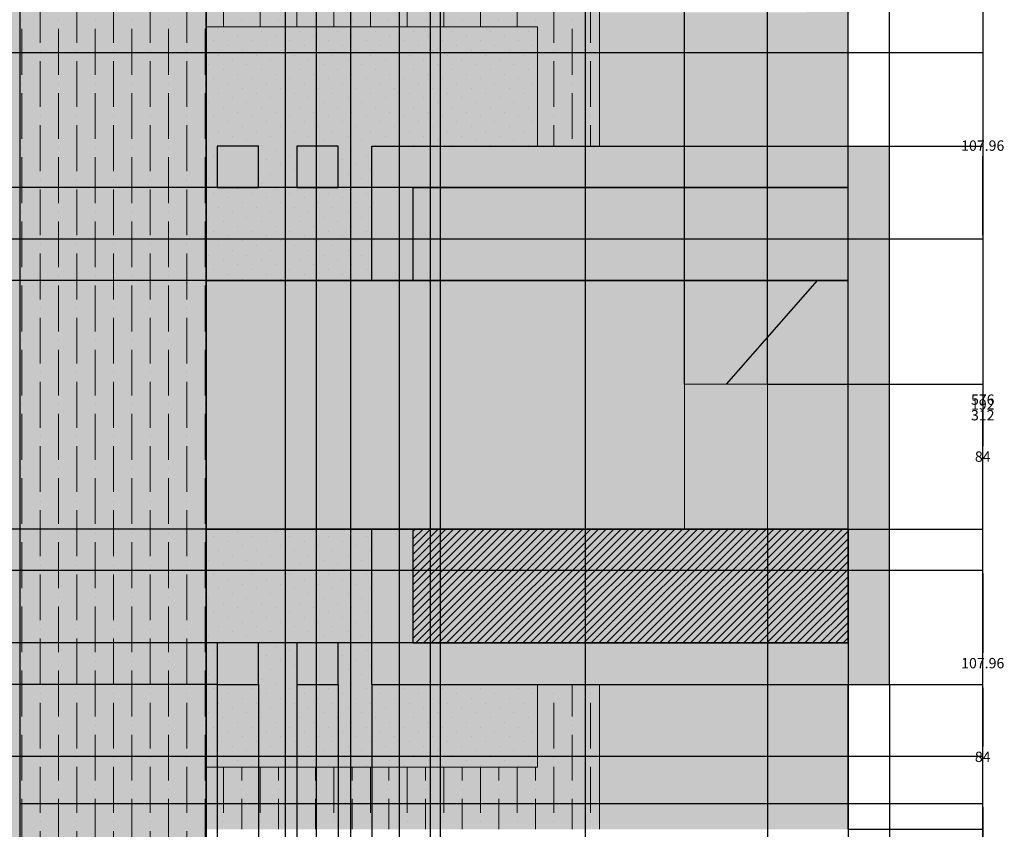
# Model space of a CAD drawing. Units: inches. Extents: x 180 to 1069, y 71 to 1267.
# Tile 7 of 8: x 498 to 1069, y 474 to 943. Entities that reach past the tile are written whole.
import ezdxf

# ---------------------------------------------------------------- set-up
doc = ezdxf.new("R2010")
doc.units = ezdxf.units.IN
doc.header["$MEASUREMENT"] = 0
for name, color, linetype, lineweight in [('A-ANNO-DIMS', 2, 'Continuous', 18), ('A-DOOR', 7, 'Continuous', 20), ('A-DOOR-PANL-PATT', 25, 'Continuous', 13), ('A-ELEV-FRAM', 7, 'Continuous', 25), ('A-RAIL-GLAS-DIAG-PATT', 140, 'Continuous', 13), ('A-WALL', 7, 'Continuous', 30), ('A-WALL-CLAD', 7, 'Continuous', 18), ('A-WALL-SCRN-JNTS-PATT', 8, 'Continuous', 13)]:
    doc.layers.add(name, color=color, linetype=linetype, lineweight=lineweight)
for name, color, linetype, lineweight, true_color in [('A-ELEV-BAND-PATT', 30, 'Continuous', 13, 0xf26722), ('A-ELEV-FRAM-PATT', 53, 'Continuous', 13, 0xefd648), ('A-ELEV-REVL-PATT', 9, 'Continuous', 13, 0xc7c8ca), ('A-RAIL-GLAS-PATT', 253, 'Continuous', 13, 0x9f9f8e), ('A-WALL-PANL-PATT', 252, 'Continuous', 13, 0x939598), ('A-WALL-PATT', 253, 'Continuous', 13, 0x9f9f8e), ('A-WALL-SCRN-PATT', 251, 'Continuous', 13, 0x636466), ('A-WALL-STUC-PATT', 9, 'Continuous', 13, 0xc7c8ca)]:
    doc.layers.add(name, color=color, linetype=linetype, lineweight=lineweight, true_color=true_color)
doc.styles.get("Standard").update_dxf_attribs({"font": 'arial.ttf'})
doc.dimstyles.get("Standard").update_dxf_attribs({"dimtxt": 6, "dimasz": 2, "dimexe": 0.18, "dimexo": 0.0625, "dimgap": 3, "dimtad": 0, "dimtih": 1, "dimtoh": 1, "dimdec": 0, "dimzin": 0, "dimdsep": 46, "dimlunit": 3, "dimtxsty": 'Standard', "dimcen": 0.09, "dimadec": 0, "dimazin": 0, "dimtfac": 1, "dimtdec": 0, "dimtofl": 0, "dimtmove": 0, "dimatfit": 3, "dimfxl": 1, "dimtolj": 1, "dimtzin": 0, "dimarcsym": 0})

# ---------------------------------------------------------------- blocks, each defined once
blk = doc.blocks.new('FACADE-SQUARE-INSET')
blk.add_lwpolyline([(24, 24), (0, 24), (0, 0), (24, 0)], close=True)
blk = doc.blocks.new('*D38')
at = {"layer": 'A-ANNO-DIMS', "color": 0, "lineweight": -2, "transparency": 16777216}
for p, q in [((978.15, 473.82), (1056.28, 473.82)), ((1056.1, 471.82), (1056.1, 415.94)), ((1056.1, 348.05), (1056.1, 403.92)), ((978.15, 346.05), (1056.28, 346.05))]:
    blk.add_line(p, q, dxfattribs=at)
at = {"layer": 'A-ANNO-DIMS', "color": 0, "transparency": 16777216}
for points in [[(1055.77, 471.82), (1056.43, 471.82), (1056.1, 473.82)], [(1055.77, 348.05), (1056.43, 348.05), (1056.1, 346.05)]]:
    blk.add_solid(points, dxfattribs=at)
at = {"layer": 'Defpoints', "color": 0, "transparency": 16777216}
for p in [(978.09, 473.82), (1056.1, 473.82), (978.09, 346.05)]:
    blk.add_point(p, dxfattribs=at)
at = {"layer": 'A-ANNO-DIMS', "color": 0, "transparency": 16777216, "insert": (1056.1, 409.93), "char_height": 6, "attachment_point": 5}
blk.add_mtext('\\A1;127.77', dxfattribs=at)
blk = doc.blocks.new('*D40')
at = {"layer": 'A-ANNO-DIMS', "color": 0, "lineweight": -2, "transparency": 16777216}
for p, q in [((652.09, 338.11), (652.09, 1263.01)), ((654.09, 1262.83), (686.8, 1262.83)), ((734.09, 1262.83), (701.38, 1262.83)), ((736.09, 338.11), (736.09, 1263.01))]:
    blk.add_line(p, q, dxfattribs=at)
at = {"layer": 'A-ANNO-DIMS', "color": 0, "transparency": 16777216}
for points in [[(654.09, 1263.16), (654.09, 1262.5), (652.09, 1262.83)], [(734.09, 1263.16), (734.09, 1262.5), (736.09, 1262.83)]]:
    blk.add_solid(points, dxfattribs=at)
at = {"layer": 'Defpoints', "color": 0, "transparency": 16777216}
for p in [(736.09, 1262.83), (652.09, 338.05), (736.09, 338.05)]:
    blk.add_point(p, dxfattribs=at)
at = {"layer": 'A-ANNO-DIMS', "color": 0, "transparency": 16777216, "insert": (694.09, 1262.83), "char_height": 6, "attachment_point": 5}
blk.add_mtext('\\A1;84', dxfattribs=at)
blk = doc.blocks.new('*D42')
at = {"layer": 'A-ANNO-DIMS', "color": 0, "lineweight": -2, "transparency": 16777216}
for p, q in [((670.09, 301.11), (670.09, 1263.01)), ((672.09, 1262.83), (686.66, 1262.83)), ((716.09, 1262.83), (701.51, 1262.83)), ((718.09, 301.11), (718.09, 1263.01))]:
    blk.add_line(p, q, dxfattribs=at)
at = {"layer": 'A-ANNO-DIMS', "color": 0, "transparency": 16777216}
for points in [[(672.09, 1263.16), (672.09, 1262.5), (670.09, 1262.83)], [(716.09, 1263.16), (716.09, 1262.5), (718.09, 1262.83)]]:
    blk.add_solid(points, dxfattribs=at)
at = {"layer": 'Defpoints', "color": 0, "transparency": 16777216}
for p in [(718.09, 1262.83), (670.09, 301.05), (718.09, 301.05)]:
    blk.add_point(p, dxfattribs=at)
at = {"layer": 'A-ANNO-DIMS', "color": 0, "transparency": 16777216, "insert": (694.09, 1262.83), "char_height": 6, "attachment_point": 5}
blk.add_mtext('\\A1;48', dxfattribs=at)
blk = doc.blocks.new('*D44')
at = {"layer": 'A-ANNO-DIMS', "color": 0, "lineweight": -2, "transparency": 16777216}
for p, q in [((606.09, 442.3), (606.09, 1263.01)), ((608.09, 1262.83), (635.5, 1262.83)), ((688, 1262.83), (660.59, 1262.83)), ((690, 442.3), (690, 1263.01))]:
    blk.add_line(p, q, dxfattribs=at)
at = {"layer": 'A-ANNO-DIMS', "color": 0, "transparency": 16777216}
for points in [[(608.09, 1263.16), (608.09, 1262.5), (606.09, 1262.83)], [(688, 1263.16), (688, 1262.5), (690, 1262.83)]]:
    blk.add_solid(points, dxfattribs=at)
at = {"layer": 'Defpoints', "color": 0, "transparency": 16777216}
for p in [(690, 1262.83), (606.09, 442.24), (690, 442.24)]:
    blk.add_point(p, dxfattribs=at)
at = {"layer": 'A-ANNO-DIMS', "color": 0, "transparency": 16777216, "insert": (648.04, 1262.83), "char_height": 6, "attachment_point": 5}
blk.add_mtext('\\A1;83.91', dxfattribs=at)
blk = doc.blocks.new('*D45')
at = {"layer": 'A-ANNO-DIMS', "color": 0, "lineweight": -2, "transparency": 16777216}
for p, q in [((690, 442.3), (690, 1263.01)), ((692, 1262.83), (702.82, 1262.83)), ((739.89, 1262.83), (729.08, 1262.83)), ((741.89, 442.3), (741.89, 1263.01))]:
    blk.add_line(p, q, dxfattribs=at)
at = {"layer": 'A-ANNO-DIMS', "color": 0, "transparency": 16777216}
for points in [[(692, 1263.16), (692, 1262.5), (690, 1262.83)], [(739.89, 1263.16), (739.89, 1262.5), (741.89, 1262.83)]]:
    blk.add_solid(points, dxfattribs=at)
at = {"layer": 'Defpoints', "color": 0, "transparency": 16777216}
for p in [(741.89, 1262.83), (690, 442.24), (741.89, 442.24)]:
    blk.add_point(p, dxfattribs=at)
at = {"layer": 'A-ANNO-DIMS', "color": 0, "transparency": 16777216, "insert": (715.95, 1262.83), "char_height": 6, "attachment_point": 5}
blk.add_mtext('\\A1;51.89', dxfattribs=at)
blk = doc.blocks.new('*D46')
at = {"layer": 'A-ANNO-DIMS', "color": 0, "lineweight": -2, "transparency": 16777216}
for p, q in [((741.89, 442.3), (741.89, 1263.01)), ((743.89, 1262.83), (776.6, 1262.83)), ((823.89, 1262.83), (791.18, 1262.83)), ((825.89, 442.3), (825.89, 1263.01))]:
    blk.add_line(p, q, dxfattribs=at)
at = {"layer": 'A-ANNO-DIMS', "color": 0, "transparency": 16777216}
for points in [[(743.89, 1263.16), (743.89, 1262.5), (741.89, 1262.83)], [(823.89, 1263.16), (823.89, 1262.5), (825.89, 1262.83)]]:
    blk.add_solid(points, dxfattribs=at)
at = {"layer": 'Defpoints', "color": 0, "transparency": 16777216}
for p in [(825.89, 1262.83), (741.89, 442.24), (825.89, 442.24)]:
    blk.add_point(p, dxfattribs=at)
at = {"layer": 'A-ANNO-DIMS', "color": 0, "transparency": 16777216, "insert": (783.89, 1262.83), "char_height": 6, "attachment_point": 5}
blk.add_mtext('\\A1;84', dxfattribs=at)
blk = doc.blocks.new('*D53')
at = {"layer": 'A-ANNO-DIMS', "color": 0, "lineweight": -2, "transparency": 16777216}
for p, q in [((438.15, 624.07), (1056.28, 624.07)), ((1056.1, 622.07), (1056.1, 576.16)), ((1056.1, 518.12), (1056.1, 564.03)), ((467.25, 516.12), (1056.28, 516.12))]:
    blk.add_line(p, q, dxfattribs=at)
at = {"layer": 'A-ANNO-DIMS', "color": 0, "transparency": 16777216}
for points in [[(1055.77, 622.07), (1056.43, 622.07), (1056.1, 624.07)], [(1055.77, 518.12), (1056.43, 518.12), (1056.1, 516.12)]]:
    blk.add_solid(points, dxfattribs=at)
at = {"layer": 'Defpoints', "color": 0, "transparency": 16777216}
for p in [(438.09, 624.07), (1056.1, 624.07), (467.19, 516.12)]:
    blk.add_point(p, dxfattribs=at)
at = {"layer": 'A-ANNO-DIMS', "color": 0, "transparency": 16777216, "insert": (1056.1, 570.1), "char_height": 6, "attachment_point": 5}
blk.add_mtext('\\A1;107.96', dxfattribs=at)
blk = doc.blocks.new('*D54')
at = {"layer": 'A-ANNO-DIMS', "color": 0, "lineweight": -2, "transparency": 16777216}
for p, q in [((438.15, 816.07), (1056.28, 816.07)), ((1056.1, 814.07), (1056.1, 726.14)), ((1056.1, 626.07), (1056.1, 714.01)), ((438.15, 624.07), (1056.28, 624.07))]:
    blk.add_line(p, q, dxfattribs=at)
at = {"layer": 'A-ANNO-DIMS', "color": 0, "transparency": 16777216}
for points in [[(1055.77, 814.07), (1056.43, 814.07), (1056.1, 816.07)], [(1055.77, 626.07), (1056.43, 626.07), (1056.1, 624.07)]]:
    blk.add_solid(points, dxfattribs=at)
at = {"layer": 'Defpoints', "color": 0, "transparency": 16777216}
for p in [(438.09, 816.07), (1056.1, 816.07), (438.09, 624.07)]:
    blk.add_point(p, dxfattribs=at)
at = {"layer": 'A-ANNO-DIMS', "color": 0, "transparency": 16777216, "insert": (1056.1, 720.07), "char_height": 6, "attachment_point": 5}
blk.add_mtext('\\A1;192', dxfattribs=at)
blk = doc.blocks.new('*D55')
at = {"layer": 'A-ANNO-DIMS', "color": 0, "lineweight": -2, "transparency": 16777216}
for p, q in [((467.25, 924.03), (1056.28, 924.03)), ((1056.1, 922.03), (1056.1, 876.12)), ((1056.1, 818.07), (1056.1, 863.99)), ((438.15, 816.07), (1056.28, 816.07))]:
    blk.add_line(p, q, dxfattribs=at)
at = {"layer": 'A-ANNO-DIMS', "color": 0, "transparency": 16777216}
for points in [[(1055.77, 922.03), (1056.43, 922.03), (1056.1, 924.03)], [(1055.77, 818.07), (1056.43, 818.07), (1056.1, 816.07)]]:
    blk.add_solid(points, dxfattribs=at)
at = {"layer": 'Defpoints', "color": 0, "transparency": 16777216}
for p in [(467.19, 924.03), (1056.1, 924.03), (438.09, 816.07)]:
    blk.add_point(p, dxfattribs=at)
at = {"layer": 'A-ANNO-DIMS', "color": 0, "transparency": 16777216, "insert": (1056.1, 870.05), "char_height": 6, "attachment_point": 5}
blk.add_mtext('\\A1;107.96', dxfattribs=at)
blk = doc.blocks.new('*D58')
at = {"layer": 'A-ANNO-DIMS', "color": 0, "lineweight": -2, "transparency": 16777216}
for p, q in [((606.09, 1010.75), (606.09, 74.62)), ((498.09, 956.75), (498.09, 74.62)), ((500.09, 74.8), (542.74, 74.8)), ((604.09, 74.8), (561.44, 74.8))]:
    blk.add_line(p, q, dxfattribs=at)
at = {"layer": 'A-ANNO-DIMS', "color": 0, "transparency": 16777216}
for points in [[(500.09, 75.14), (500.09, 74.47), (498.09, 74.8)], [(604.09, 75.14), (604.09, 74.47), (606.09, 74.8)]]:
    blk.add_solid(points, dxfattribs=at)
at = {"layer": 'Defpoints', "color": 0, "transparency": 16777216}
for p in [(606.09, 1010.82), (498.09, 956.82), (606.09, 74.8)]:
    blk.add_point(p, dxfattribs=at)
at = {"layer": 'A-ANNO-DIMS', "color": 0, "transparency": 16777216, "insert": (552.09, 74.8), "char_height": 6, "attachment_point": 5}
blk.add_mtext('\\A1;108', dxfattribs=at)
blk = doc.blocks.new('*D59')
at = {"layer": 'A-ANNO-DIMS', "color": 0, "lineweight": -2, "transparency": 16777216}
for p, q in [((606.15, 1010.82), (1056.28, 1010.82)), ((1056.1, 1008.82), (1056.1, 728.88)), ((1056.1, 436.82), (1056.1, 716.75)), ((606.15, 434.82), (1056.28, 434.82))]:
    blk.add_line(p, q, dxfattribs=at)
at = {"layer": 'A-ANNO-DIMS', "color": 0, "transparency": 16777216}
for points in [[(1055.77, 1008.82), (1056.43, 1008.82), (1056.1, 1010.82)], [(1055.77, 436.82), (1056.43, 436.82), (1056.1, 434.82)]]:
    blk.add_solid(points, dxfattribs=at)
at = {"layer": 'Defpoints', "color": 0, "transparency": 16777216}
for p in [(606.09, 1010.82), (1056.1, 1010.82), (606.09, 434.82)]:
    blk.add_point(p, dxfattribs=at)
at = {"layer": 'A-ANNO-DIMS', "color": 0, "transparency": 16777216, "insert": (1056.1, 722.82), "char_height": 6, "attachment_point": 5}
blk.add_mtext('\\A1;576', dxfattribs=at)
blk = doc.blocks.new('*D60')
at = {"layer": 'A-ANNO-DIMS', "color": 0, "lineweight": -2, "transparency": 16777216}
for p, q in [((498.15, 488.82), (1056.28, 488.82)), ((1056.1, 486.82), (1056.1, 467.87)), ((1056.1, 436.82), (1056.1, 455.76)), ((606.15, 434.82), (1056.28, 434.82))]:
    blk.add_line(p, q, dxfattribs=at)
at = {"layer": 'A-ANNO-DIMS', "color": 0, "transparency": 16777216}
for points in [[(1055.77, 486.82), (1056.43, 486.82), (1056.1, 488.82)], [(1055.77, 436.82), (1056.43, 436.82), (1056.1, 434.82)]]:
    blk.add_solid(points, dxfattribs=at)
at = {"layer": 'Defpoints', "color": 0, "transparency": 16777216}
for p in [(498.09, 488.82), (606.09, 434.82), (1056.1, 434.82)]:
    blk.add_point(p, dxfattribs=at)
at = {"layer": 'A-ANNO-DIMS', "color": 0, "transparency": 16777216, "insert": (1056.1, 461.82), "char_height": 6, "attachment_point": 5}
blk.add_mtext('\\A1;54', dxfattribs=at)
blk = doc.blocks.new('*D64')
at = {"layer": 'A-ANNO-DIMS', "color": 0, "lineweight": -2, "transparency": 16777216}
for p, q in [((612.46, 845.82), (191.89, 845.82)), ((192.07, 843.82), (192.07, 707.88)), ((192.07, 559.82), (192.07, 695.75)), ((612.46, 557.82), (191.89, 557.82))]:
    blk.add_line(p, q, dxfattribs=at)
at = {"layer": 'A-ANNO-DIMS', "color": 0, "transparency": 16777216}
for points in [[(191.74, 843.82), (192.41, 843.82), (192.07, 845.82)], [(191.74, 559.82), (192.41, 559.82), (192.07, 557.82)]]:
    blk.add_solid(points, dxfattribs=at)
at = {"layer": 'Defpoints', "color": 0, "transparency": 16777216}
for p in [(192.07, 845.82), (612.53, 845.82), (612.53, 557.82)]:
    blk.add_point(p, dxfattribs=at)
at = {"layer": 'A-ANNO-DIMS', "color": 0, "transparency": 16777216, "insert": (192.07, 701.82), "char_height": 6, "attachment_point": 5}
blk.add_mtext('\\A1;288', dxfattribs=at)
blk = doc.blocks.new('*D65')
at = {"layer": 'A-ANNO-DIMS', "color": 0, "lineweight": -2, "transparency": 16777216}
for p, q in [((636.53, 557.75), (636.53, 74.62)), ((658.66, 557.75), (658.66, 74.62)), ((638.53, 74.8), (656.66, 74.8)), ((658.66, 74.8), (660.66, 74.8))]:
    blk.add_line(p, q, dxfattribs=at)
at = {"layer": 'A-ANNO-DIMS', "color": 0, "transparency": 16777216}
for points in [[(638.53, 75.14), (638.53, 74.47), (636.53, 74.8)], [(656.66, 75.14), (656.66, 74.47), (658.66, 74.8)]]:
    blk.add_solid(points, dxfattribs=at)
at = {"layer": 'Defpoints', "color": 0, "transparency": 16777216}
for p in [(636.53, 557.82), (658.66, 557.82), (658.66, 74.8)]:
    blk.add_point(p, dxfattribs=at)
at = {"layer": 'A-ANNO-DIMS', "color": 0, "transparency": 16777216, "insert": (676.17, 74.8), "char_height": 6, "attachment_point": 5}
blk.add_mtext('\\A1;22.133', dxfattribs=at)
blk = doc.blocks.new('*D66')
at = {"layer": 'A-ANNO-DIMS', "color": 0, "lineweight": -2, "transparency": 16777216}
for p, q in [((606.09, 647.75), (606.09, 74.62)), ((612.53, 557.75), (612.53, 74.62)), ((604.09, 74.8), (602.09, 74.8)), ((614.53, 74.8), (616.53, 74.8))]:
    blk.add_line(p, q, dxfattribs=at)
at = {"layer": 'A-ANNO-DIMS', "color": 0, "transparency": 16777216}
for points in [[(604.09, 75.14), (604.09, 74.47), (606.09, 74.8)], [(614.53, 75.14), (614.53, 74.47), (612.53, 74.8)]]:
    blk.add_solid(points, dxfattribs=at)
at = {"layer": 'Defpoints', "color": 0, "transparency": 16777216}
for p in [(606.09, 647.82), (612.53, 557.82), (612.53, 74.8)]:
    blk.add_point(p, dxfattribs=at)
at = {"layer": 'A-ANNO-DIMS', "color": 0, "transparency": 16777216, "insert": (627.32, 74.8), "char_height": 6, "attachment_point": 5}
blk.add_mtext('\\A1;6.44', dxfattribs=at)
blk = doc.blocks.new('*D67')
at = {"layer": 'A-ANNO-DIMS', "color": 0, "lineweight": -2, "transparency": 16777216}
for p, q in [((682.66, 557.75), (682.66, 74.62)), ((702.09, 557.75), (702.09, 74.62)), ((684.66, 74.8), (700.09, 74.8)), ((702.09, 74.8), (704.09, 74.8))]:
    blk.add_line(p, q, dxfattribs=at)
at = {"layer": 'A-ANNO-DIMS', "color": 0, "transparency": 16777216}
for points in [[(684.66, 75.14), (684.66, 74.47), (682.66, 74.8)], [(700.09, 75.14), (700.09, 74.47), (702.09, 74.8)]]:
    blk.add_solid(points, dxfattribs=at)
at = {"layer": 'Defpoints', "color": 0, "transparency": 16777216}
for p in [(682.66, 557.82), (702.09, 557.82), (702.09, 74.8)]:
    blk.add_point(p, dxfattribs=at)
at = {"layer": 'A-ANNO-DIMS', "color": 0, "transparency": 16777216, "insert": (719.26, 74.8), "char_height": 6, "attachment_point": 5}
blk.add_mtext('\\A1;19.427', dxfattribs=at)
blk = doc.blocks.new('*D68')
at = {"layer": 'A-ANNO-DIMS', "color": 0, "lineweight": -2, "transparency": 16777216}
for p, q in [((702.09, 557.75), (702.09, 74.62)), ((1002.09, 557.75), (1002.09, 74.62)), ((704.09, 74.8), (842.47, 74.8)), ((1000.09, 74.8), (861.7, 74.8))]:
    blk.add_line(p, q, dxfattribs=at)
at = {"layer": 'A-ANNO-DIMS', "color": 0, "transparency": 16777216}
for points in [[(704.09, 75.14), (704.09, 74.47), (702.09, 74.8)], [(1000.09, 75.14), (1000.09, 74.47), (1002.09, 74.8)]]:
    blk.add_solid(points, dxfattribs=at)
at = {"layer": 'Defpoints', "color": 0, "transparency": 16777216}
for p in [(702.09, 557.82), (1002.09, 557.82), (1002.09, 74.8)]:
    blk.add_point(p, dxfattribs=at)
at = {"layer": 'A-ANNO-DIMS', "color": 0, "transparency": 16777216, "insert": (852.09, 74.8), "char_height": 6, "attachment_point": 5}
blk.add_mtext('\\A1;300', dxfattribs=at)
blk = doc.blocks.new('*D69')
at = {"layer": 'A-ANNO-DIMS', "color": 0, "lineweight": -2, "transparency": 16777216}
for p, q in [((1002.15, 557.82), (1056.28, 557.82)), ((1056.1, 555.82), (1056.1, 521.88)), ((1056.1, 475.82), (1056.1, 509.75)), ((978.15, 473.82), (1056.28, 473.82))]:
    blk.add_line(p, q, dxfattribs=at)
at = {"layer": 'A-ANNO-DIMS', "color": 0, "transparency": 16777216}
for points in [[(1055.77, 555.82), (1056.43, 555.82), (1056.1, 557.82)], [(1055.77, 475.82), (1056.43, 475.82), (1056.1, 473.82)]]:
    blk.add_solid(points, dxfattribs=at)
at = {"layer": 'Defpoints', "color": 0, "transparency": 16777216}
for p in [(1002.09, 557.82), (1056.1, 557.82), (978.09, 473.82)]:
    blk.add_point(p, dxfattribs=at)
at = {"layer": 'A-ANNO-DIMS', "color": 0, "transparency": 16777216, "insert": (1056.1, 515.82), "char_height": 6, "attachment_point": 5}
blk.add_mtext('\\A1;84', dxfattribs=at)
blk = doc.blocks.new('*D70')
at = {"layer": 'A-ANNO-DIMS', "color": 0, "lineweight": -2, "transparency": 16777216}
for p, q in [((1002.15, 869.82), (1056.28, 869.82)), ((1056.1, 867.82), (1056.1, 719.88)), ((1056.1, 559.82), (1056.1, 707.75)), ((1002.15, 557.82), (1056.28, 557.82))]:
    blk.add_line(p, q, dxfattribs=at)
at = {"layer": 'A-ANNO-DIMS', "color": 0, "transparency": 16777216}
for points in [[(1055.77, 867.82), (1056.43, 867.82), (1056.1, 869.82)], [(1055.77, 559.82), (1056.43, 559.82), (1056.1, 557.82)]]:
    blk.add_solid(points, dxfattribs=at)
at = {"layer": 'Defpoints', "color": 0, "transparency": 16777216}
for p in [(1002.09, 869.82), (1056.1, 869.82), (1002.09, 557.82)]:
    blk.add_point(p, dxfattribs=at)
at = {"layer": 'A-ANNO-DIMS', "color": 0, "transparency": 16777216, "insert": (1056.1, 713.82), "char_height": 6, "attachment_point": 5}
blk.add_mtext('\\A1;312', dxfattribs=at)
blk = doc.blocks.new('*D71')
at = {"layer": 'A-ANNO-DIMS', "color": 0, "lineweight": -2, "transparency": 16777216}
for p, q in [((978.02, 647.82), (191.89, 647.82)), ((192.07, 645.82), (192.07, 620.88)), ((192.07, 583.82), (192.07, 608.75)), ((978.02, 581.82), (191.89, 581.82))]:
    blk.add_line(p, q, dxfattribs=at)
at = {"layer": 'A-ANNO-DIMS', "color": 0, "transparency": 16777216}
for points in [[(191.74, 645.82), (192.41, 645.82), (192.07, 647.82)], [(191.74, 583.82), (192.41, 583.82), (192.07, 581.82)]]:
    blk.add_solid(points, dxfattribs=at)
at = {"layer": 'Defpoints', "color": 0, "transparency": 16777216}
for p in [(192.07, 647.82), (978.09, 647.82), (978.09, 581.82)]:
    blk.add_point(p, dxfattribs=at)
at = {"layer": 'A-ANNO-DIMS', "color": 0, "transparency": 16777216, "insert": (192.07, 614.82), "char_height": 6, "attachment_point": 5}
blk.add_mtext('\\A1;66', dxfattribs=at)
blk = doc.blocks.new('*D72')
at = {"layer": 'A-ANNO-DIMS', "color": 0, "lineweight": -2, "transparency": 16777216}
for p, q in [((978.02, 791.82), (191.89, 791.82)), ((192.07, 789.82), (192.07, 725.83)), ((192.07, 649.82), (192.07, 713.8)), ((978.02, 647.82), (191.89, 647.82))]:
    blk.add_line(p, q, dxfattribs=at)
at = {"layer": 'A-ANNO-DIMS', "color": 0, "transparency": 16777216}
for points in [[(191.74, 789.82), (192.41, 789.82), (192.07, 791.82)], [(191.74, 649.82), (192.41, 649.82), (192.07, 647.82)]]:
    blk.add_solid(points, dxfattribs=at)
at = {"layer": 'Defpoints', "color": 0, "transparency": 16777216}
for p in [(192.07, 791.82), (978.09, 791.82), (978.09, 647.82)]:
    blk.add_point(p, dxfattribs=at)
at = {"layer": 'A-ANNO-DIMS', "color": 0, "transparency": 16777216, "insert": (192.07, 719.82), "char_height": 6, "attachment_point": 5}
blk.add_mtext('\\A1;144', dxfattribs=at)
blk = doc.blocks.new('*D73')
at = {"layer": 'A-ANNO-DIMS', "color": 0, "lineweight": -2, "transparency": 16777216}
for p, q in [((978.02, 845.82), (191.89, 845.82)), ((192.07, 843.82), (192.07, 824.87)), ((192.07, 793.82), (192.07, 812.76)), ((978.02, 791.82), (191.89, 791.82))]:
    blk.add_line(p, q, dxfattribs=at)
at = {"layer": 'A-ANNO-DIMS', "color": 0, "transparency": 16777216}
for points in [[(191.74, 843.82), (192.41, 843.82), (192.07, 845.82)], [(191.74, 793.82), (192.41, 793.82), (192.07, 791.82)]]:
    blk.add_solid(points, dxfattribs=at)
at = {"layer": 'Defpoints', "color": 0, "transparency": 16777216}
for p in [(192.07, 845.82), (978.09, 845.82), (978.09, 791.82)]:
    blk.add_point(p, dxfattribs=at)
at = {"layer": 'A-ANNO-DIMS', "color": 0, "transparency": 16777216, "insert": (192.07, 818.82), "char_height": 6, "attachment_point": 5}
blk.add_mtext('\\A1;54', dxfattribs=at)
blk = doc.blocks.new('*D74')
at = {"layer": 'A-ANNO-DIMS', "color": 0, "lineweight": -2, "transparency": 16777216}
for p, q in [((976.09, 1262.83), (974.09, 1262.83)), ((978.09, 845.88), (978.09, 1263.01)), ((1002.09, 869.88), (1002.09, 1263.01)), ((1004.09, 1262.83), (1006.09, 1262.83))]:
    blk.add_line(p, q, dxfattribs=at)
at = {"layer": 'A-ANNO-DIMS', "color": 0, "transparency": 16777216}
for points in [[(976.09, 1263.16), (976.09, 1262.5), (978.09, 1262.83)], [(1004.09, 1263.16), (1004.09, 1262.5), (1002.09, 1262.83)]]:
    blk.add_solid(points, dxfattribs=at)
at = {"layer": 'Defpoints', "color": 0, "transparency": 16777216}
for p in [(1002.09, 1262.83), (1002.09, 869.82), (978.09, 845.82)]:
    blk.add_point(p, dxfattribs=at)
at = {"layer": 'A-ANNO-DIMS', "color": 0, "transparency": 16777216, "insert": (990.09, 1262.83), "char_height": 6, "attachment_point": 5}
blk.add_mtext('\\A1;24', dxfattribs=at)
blk = doc.blocks.new('*D77')
at = {"layer": 'A-ANNO-DIMS', "color": 0, "lineweight": -2, "transparency": 16777216}
for p, q in [((883.35, 731.88), (883.35, 1263.01)), ((885.35, 1262.83), (899.93, 1262.83)), ((929.35, 1262.83), (914.78, 1262.83)), ((931.35, 731.88), (931.35, 1263.01))]:
    blk.add_line(p, q, dxfattribs=at)
at = {"layer": 'A-ANNO-DIMS', "color": 0, "transparency": 16777216}
for points in [[(885.35, 1263.16), (885.35, 1262.5), (883.35, 1262.83)], [(929.35, 1263.16), (929.35, 1262.5), (931.35, 1262.83)]]:
    blk.add_solid(points, dxfattribs=at)
at = {"layer": 'Defpoints', "color": 0, "transparency": 16777216}
for p in [(931.35, 1262.83), (883.35, 731.82), (931.35, 731.82)]:
    blk.add_point(p, dxfattribs=at)
at = {"layer": 'A-ANNO-DIMS', "color": 0, "transparency": 16777216, "insert": (907.35, 1262.83), "char_height": 6, "attachment_point": 5}
blk.add_mtext('\\A1;48', dxfattribs=at)
blk = doc.blocks.new('*D78')
at = {"layer": 'A-ANNO-DIMS', "color": 0, "lineweight": -2, "transparency": 16777216}
for p, q in [((931.41, 731.82), (1056.28, 731.82)), ((1056.1, 729.82), (1056.1, 695.88)), ((1056.1, 649.82), (1056.1, 683.75)), ((931.41, 647.82), (1056.28, 647.82))]:
    blk.add_line(p, q, dxfattribs=at)
at = {"layer": 'A-ANNO-DIMS', "color": 0, "transparency": 16777216}
for points in [[(1055.77, 729.82), (1056.43, 729.82), (1056.1, 731.82)], [(1055.77, 649.82), (1056.43, 649.82), (1056.1, 647.82)]]:
    blk.add_solid(points, dxfattribs=at)
at = {"layer": 'Defpoints', "color": 0, "transparency": 16777216}
for p in [(931.35, 731.82), (1056.1, 731.82), (931.35, 647.82)]:
    blk.add_point(p, dxfattribs=at)
at = {"layer": 'A-ANNO-DIMS', "color": 0, "transparency": 16777216, "insert": (1056.1, 689.82), "char_height": 6, "attachment_point": 5}
blk.add_mtext('\\A1;84', dxfattribs=at)
blk = doc.blocks.new('*D79')
at = {"layer": 'A-ANNO-DIMS', "color": 0, "lineweight": -2, "transparency": 16777216}
for p, q in [((931.35, 647.75), (931.35, 74.62)), ((978.09, 647.75), (978.09, 74.62)), ((933.35, 74.8), (941.49, 74.8)), ((976.09, 74.8), (967.95, 74.8))]:
    blk.add_line(p, q, dxfattribs=at)
at = {"layer": 'A-ANNO-DIMS', "color": 0, "transparency": 16777216}
for points in [[(933.35, 75.14), (933.35, 74.47), (931.35, 74.8)], [(976.09, 75.14), (976.09, 74.47), (978.09, 74.8)]]:
    blk.add_solid(points, dxfattribs=at)
at = {"layer": 'Defpoints', "color": 0, "transparency": 16777216}
for p in [(931.35, 647.82), (978.09, 647.82), (978.09, 74.8)]:
    blk.add_point(p, dxfattribs=at)
at = {"layer": 'A-ANNO-DIMS', "color": 0, "transparency": 16777216, "insert": (954.72, 74.8), "char_height": 6, "attachment_point": 5}
blk.add_mtext('\\A1;46.74', dxfattribs=at)

msp = doc.modelspace()

# ---------------------------------------------------------------- hatches: boundary and pattern name
at = {"layer": 'A-DOOR-PANL-PATT'}
h = msp.add_hatch(color=256, dxfattribs=at)
h.dxf.hatch_style = 1
h.paths.add_polyline_path([(931.3511, 731.8159), (883.3511, 731.8159), (883.3511, 647.8159), (931.3511, 647.8159)])
at = {"layer": 'A-ELEV-BAND-PATT'}
h = msp.add_hatch(color=256, dxfattribs=at)
h.dxf.hatch_style = 1
h.paths.add_polyline_path([(1002.0875, 1148.8159), (726.0875, 1148.8159), (726.0875, 1130.8159), (954.0875, 1130.8159), (954.0875, 947.2513), (978.0875, 947.2513), (978.0875, 1130.8159), (1002.0875, 1130.8159)])
h.paths.add_polyline_path([(654.0875, 1148.8159), (354.0875, 1148.8159), (354.0875, 1130.8159), (654.0875, 1130.8159)])
h.paths.add_polyline_path([(606.0875, 434.8159), (246.0875, 434.8159), (246.0875, 416.8159), (606.0875, 416.8159)])
h.paths.add_polyline_path([(978.0875, 845.8159), (726.0875, 845.8159), (726.0875, 791.8159), (978.0875, 791.8159)])
at = {"layer": 'A-ELEV-FRAM-PATT'}
h = msp.add_hatch(color=256, dxfattribs=at)
h.dxf.hatch_style = 1
h.paths.add_polyline_path([(354.0875, 1184.8159), (654.0875, 1184.8159), (654.0875, 974.8159), (726.0875, 974.8159), (726.0875, 1208.8159), (288.0875, 1208.8159), (288.0875, 897.6348), (304.7188, 897.6348), (304.7188, 883.4805), (288.0875, 883.4805), (288.0875, 866.8025), (304.7188, 866.8025), (304.7188, 852.6482), (288.0875, 852.6482), (288.0875, 835.9702), (304.7188, 835.9702), (304.7188, 821.8159), (288.0875, 821.8159), (288.0875, 805.1379), (304.7188, 805.1379), (304.7188, 790.9836), (288.0875, 790.9836), (288.0875, 774.3056), (304.7188, 774.3056), (304.7188, 760.1513), (288.0875, 760.1513), (288.0875, 743.4733), (304.7188, 743.4733), (304.7188, 729.319), (288.0875, 729.319), (288.0875, 434.8159), (354.0875, 434.8159), (354.0875, 456.1177), (317.1892, 456.1177), (317.1892, 516.1177), (354.0875, 516.1177), (354.0875, 924.0304), (317.1892, 924.0304), (317.1892, 984.0304), (354.0875, 984.0304)])
h.paths.add_polyline_path([(1002.0875, 869.8159), (702.0875, 869.8159), (702.0875, 791.8159), (726.0875, 791.8159), (726.0875, 845.8159), (978.0875, 845.8159), (978.0875, 581.8159), (726.0875, 581.8159), (726.0875, 647.8159), (702.0875, 647.8159), (702.0875, 557.8159), (1002.0875, 557.8159)])
h.paths.add_polyline_path([(906.0875, 1080.2003), (882.0875, 1080.2003), (882.0875, 1056.2003), (906.0875, 1056.2003)])
h.paths.add_polyline_path([(906.0875, 996.2003), (882.0875, 996.2003), (882.0875, 972.2003), (906.0875, 972.2003)])
h.paths.add_polyline_path([(636.5273, 869.8159), (612.5273, 869.8159), (612.5273, 845.8159), (636.5273, 845.8159)], flags=17)
h.paths.add_polyline_path([(682.6602, 869.8159), (658.6602, 869.8159), (658.6602, 845.8159), (682.6602, 845.8159)], flags=17)
h.paths.add_polyline_path([(636.5273, 581.8159), (612.5273, 581.8159), (612.5273, 557.8159), (636.5273, 557.8159)], flags=17)
h.paths.add_polyline_path([(682.6602, 581.8159), (658.6602, 581.8159), (658.6602, 557.8159), (682.6602, 557.8159)], flags=17)
h.paths.add_polyline_path([(942.0875, 358.0477), (918.0875, 358.0477), (918.0875, 128.8159), (942.0875, 128.8159)])
h.paths.add_polyline_path([(630.0875, 358.0477), (606.0875, 358.0477), (606.0875, 128.8159), (630.0875, 128.8159)])
at = {"layer": 'A-ELEV-REVL-PATT'}
h = msp.add_hatch(color=256, dxfattribs=at)
h.dxf.hatch_style = 1
h.paths.add_polyline_path([(978.0875, 791.8159), (960.2423, 791.8159), (907.3511, 731.8159), (931.3511, 731.8159), (931.3511, 647.8159), (978.0875, 647.8159)])
h.paths.add_polyline_path([(978.0875, 346.0477), (942.0875, 346.0477), (942.0875, 128.8159), (978.0875, 128.8159)])
at = {"layer": 'A-RAIL-GLAS-DIAG-PATT'}
h = msp.add_hatch(dxfattribs=at)
h.set_pattern_fill('ANSI31', color=256, scale=25)
h.paths.add_polyline_path([(978.0875, 647.8159), (726.0875, 647.8159), (726.0875, 581.8159), (978.0875, 581.8159)])
at = {"layer": 'A-RAIL-GLAS-PATT'}
h = msp.add_hatch(color=256, dxfattribs=at)
h.dxf.hatch_style = 1
h.paths.add_polyline_path([(978.0875, 647.8159), (726.0875, 647.8159), (726.0875, 581.8159), (978.0875, 581.8159)])
at = {"layer": 'A-WALL-PANL-PATT'}
h = msp.add_hatch(color=256, dxfattribs=at)
h.dxf.hatch_style = 1
h.paths.add_polyline_path([(498.0875, 956.8159), (467.1892, 956.8159), (467.1892, 924.0304), (354.0875, 924.0304), (354.0875, 816.0741), (438.0875, 816.0741), (438.0875, 624.0741), (354.0875, 624.0741), (354.0875, 516.1177), (467.1892, 516.1177), (467.1892, 488.8159), (498.0875, 488.8159)])
h.paths.add_polyline_path([(798.0875, 938.8159), (606.0875, 938.8159), (606.0875, 791.8159), (702.0875, 791.8159), (702.0875, 869.8159), (798.0875, 869.8159)])
h.paths.add_polyline_path([(682.6602, 869.8159), (682.6602, 845.8159), (658.6602, 845.8159), (658.6602, 869.8159)], flags=16)
h.paths.add_polyline_path([(636.5273, 869.8159), (636.5273, 845.8159), (612.5273, 845.8159), (612.5273, 869.8159)], flags=16)
h.paths.add_polyline_path([(702.0875, 647.8159), (606.0875, 647.8159), (606.0875, 509.8159), (798.0875, 509.8159), (798.0875, 557.8159), (702.0875, 557.8159)])
h.paths.add_polyline_path([(658.6602, 581.8159), (682.6602, 581.8159), (682.6602, 557.8159), (658.6602, 557.8159)], flags=16)
h.paths.add_polyline_path([(636.5273, 581.8159), (636.5273, 557.8159), (612.5273, 557.8159), (612.5273, 581.8159)], flags=16)
at = {"layer": 'A-WALL-PATT'}
h = msp.add_hatch(color=256, dxfattribs=at)
h.dxf.hatch_style = 1
h.paths.add_polyline_path([(978.0875, 947.2513), (834.0875, 947.2513), (834.0875, 869.8159), (978.0875, 869.8159)])
h.paths.add_polyline_path([(978.0875, 557.8159), (834.0875, 557.8159), (834.0875, 473.8159), (978.0875, 473.8159)])
h.paths.add_polyline_path([(960.2423, 791.8159), (606.0875, 791.8159), (606.0875, 647.8159), (883.3511, 647.8159), (883.3511, 731.8159), (907.3511, 731.8159)])
at = {"layer": 'A-WALL-SCRN-JNTS-PATT'}
h = msp.add_hatch(dxfattribs=at)
h.set_pattern_fill('ANSI36', color=256, scale=85, angle=45)
h.paths.add_polyline_path([(606.0875, 938.8159), (798.0875, 938.8159), (798.0875, 869.8159), (834.0875, 869.8159), (834.0875, 974.8159), (606.0875, 974.8159), (606.0875, 1010.8159), (354.0875, 1010.8159), (354.0875, 984.0304), (467.1892, 984.0304), (467.1892, 956.8159), (498.0875, 956.8159), (498.0875, 488.8159), (467.1892, 488.8159), (467.1892, 456.1177), (354.0875, 456.1177), (354.0875, 434.8159), (606.0875, 434.8159), (606.0875, 473.8159), (834.0875, 473.8159), (834.0875, 557.8159), (798.0875, 557.8159), (798.0875, 509.8159), (606.0875, 509.8159)])
at = {"layer": 'A-WALL-SCRN-PATT'}
h = msp.add_hatch(color=256, dxfattribs=at)
h.dxf.hatch_style = 1
h.paths.add_polyline_path([(606.0875, 938.8159), (798.0875, 938.8159), (798.0875, 869.8159), (834.0875, 869.8159), (834.0875, 974.8159), (606.0875, 974.8159), (606.0875, 1010.8159), (354.0875, 1010.8159), (354.0875, 984.0304), (467.1892, 984.0304), (467.1892, 956.8159), (498.0875, 956.8159), (498.0875, 488.8159), (467.1892, 488.8159), (467.1892, 456.1177), (354.0875, 456.1177), (354.0875, 434.8159), (606.0875, 434.8159), (606.0875, 473.8159), (834.0875, 473.8159), (834.0875, 557.8159), (798.0875, 557.8159), (798.0875, 509.8159), (606.0875, 509.8159)])
h.paths.add_polyline_path([(367.1892, 507.1177), (326.1892, 507.1177), (326.1892, 465.1177), (367.1892, 465.1177)])
h.paths.add_polyline_path([(411.1892, 507.1177), (373.1892, 507.1177), (373.1892, 465.1177), (411.1892, 465.1177)], flags=17)
h.paths.add_polyline_path([(458.1892, 507.1177), (417.1892, 507.1177), (417.1892, 465.1177), (458.1892, 465.1177)], flags=17)
h.paths.add_polyline_path([(426.0875, 672.0741), (354.0875, 672.0741), (354.0875, 636.0741), (426.0875, 636.0741)], flags=17)
h.paths.add_polyline_path([(426.0875, 760.0741), (354.0875, 760.0741), (354.0875, 680.0741), (426.0875, 680.0741)], flags=17)
h.paths.add_polyline_path([(426.0875, 804.0741), (354.0875, 804.0741), (354.0875, 768.0741), (426.0875, 768.0741)], flags=17)
h.paths.add_polyline_path([(367.1892, 975.0304), (326.1892, 975.0304), (326.1892, 933.0304), (367.1892, 933.0304)])
h.paths.add_polyline_path([(411.1892, 975.0304), (373.1892, 975.0304), (373.1892, 933.0304), (411.1892, 933.0304)], flags=17)
h.paths.add_polyline_path([(458.1892, 975.0304), (417.1892, 975.0304), (417.1892, 933.0304), (458.1892, 933.0304)], flags=17)
at = {"layer": 'A-WALL-STUC-PATT'}
h = msp.add_hatch(dxfattribs=at)
h.set_pattern_fill('DOTS', color=256, scale=125, angle=45)
h.paths.add_polyline_path([(798.0875, 938.8159), (606.0875, 938.8159), (606.0875, 791.8159), (702.0875, 791.8159), (702.0875, 869.8159), (798.0875, 869.8159)])
h.paths.add_polyline_path([(682.6602, 869.8159), (682.6602, 845.8159), (658.6602, 845.8159), (658.6602, 869.8159)], flags=16)
h.paths.add_polyline_path([(636.5273, 869.8159), (636.5273, 845.8159), (612.5273, 845.8159), (612.5273, 869.8159)], flags=16)
h.paths.add_polyline_path([(798.0875, 557.8159), (702.0875, 557.8159), (702.0875, 647.8159), (606.0875, 647.8159), (606.0875, 509.8159), (798.0875, 509.8159)])
h.paths.add_polyline_path([(682.6602, 557.8159), (658.6602, 557.8159), (658.6602, 581.8159), (682.6602, 581.8159)], flags=16)
h.paths.add_polyline_path([(636.5273, 557.8159), (612.5273, 557.8159), (612.5273, 581.8159), (636.5273, 581.8159)], flags=16)

# ---------------------------------------------------------------- linework, layer by layer
at = {"layer": 'A-DOOR'}
for p, q in [((931.3511, 731.8159), (883.3511, 731.8159)), ((883.3511, 731.8159), (883.3511, 647.8159)), ((931.3511, 647.8159), (931.3511, 731.8159))]:
    msp.add_line(p, q, dxfattribs=at)
at = {"layer": 'A-ELEV-FRAM'}
for p, q in [((702.0875, 869.8159), (1002.0875, 869.8159)), ((702.0875, 791.8159), (702.0875, 869.8159)), ((1002.0875, 557.8159), (1002.0875, 869.8159)), ((726.0875, 845.8159), (978.0875, 845.8159)), ((726.0875, 791.8159), (726.0875, 845.8159)), ((978.0875, 581.8159), (978.0875, 845.8159)), ((702.0875, 557.8159), (702.0875, 647.8159)), ((726.0875, 581.8159), (726.0875, 647.8159)), ((726.0875, 581.8159), (978.0875, 581.8159)), ((702.0875, 557.8159), (1002.0875, 557.8159))]:
    msp.add_line(p, q, dxfattribs=at)
at = {"layer": 'A-WALL'}
for p, q in [((978.0875, 869.8159), (978.0875, 1130.8159)), ((606.0875, 791.8159), (978.0875, 791.8159)), ((960.2423, 791.8159), (907.3511, 731.8159)), ((606.0875, 647.8159), (978.0875, 647.8159)), ((978.0875, 473.8159), (978.0875, 557.8159))]:
    msp.add_line(p, q, dxfattribs=at)
at = {"layer": 'A-WALL-CLAD'}
for p, q in [((834.0875, 974.8159), (834.0875, 869.8159)), ((606.0875, 938.8159), (798.0875, 938.8159)), ((606.0875, 509.8159), (606.0875, 938.8159)), ((798.0875, 938.8159), (798.0875, 869.8159)), ((798.0875, 557.8159), (798.0875, 509.8159)), ((834.0875, 557.8159), (834.0875, 473.8159)), ((606.0875, 509.8159), (798.0875, 509.8159))]:
    msp.add_line(p, q, dxfattribs=at)

# ---------------------------------------------------------------- block references
at = {"layer": 'A-ELEV-FRAM'}
for p in [(612.5273, 845.8159), (658.6602, 845.8159), (612.5273, 557.8159), (658.6602, 557.8159)]:
    msp.add_blockref('FACADE-SQUARE-INSET', p, dxfattribs=at)

# ---------------------------------------------------------------- dimensions: what is measured, and where the dimension line sits
at = {"layer": 'A-ANNO-DIMS'}
for base, p1, p2, override, picture, middle in [((690.001, 1262.8294), (606.0875, 442.2382), (690.001, 442.2382), {"dimdec": 2, "dimlfac": 1, "dimrnd": 0, "dimzin": 0, "dimdsep": 46, "dimlunit": 2}, '*D44', (648.0442, 1262.8294)), ((736.0875, 1262.8294), (652.0875, 338.0477), (736.0875, 338.0477), {"dimdec": 0, "dimlfac": 1, "dimrnd": 0, "dimzin": 0, "dimdsep": 46, "dimlunit": 2}, '*D40', (694.0875, 1262.8294)), ((718.0875, 1262.8294), (670.0875, 301.0477), (718.0875, 301.0477), {"dimdec": 0, "dimlfac": 1, "dimrnd": 0, "dimzin": 0, "dimdsep": 46, "dimlunit": 2}, '*D42', (694.0875, 1262.8294)), ((741.8928, 1262.8294), (690.001, 442.2382), (741.8928, 442.2382), {"dimdec": 2, "dimlfac": 1, "dimrnd": 0, "dimzin": 0, "dimdsep": 46, "dimlunit": 2}, '*D45', (715.9469, 1262.8294)), ((825.8928, 1262.8294), (741.8928, 442.2382), (825.8928, 442.2382), {"dimdec": 0, "dimlfac": 1, "dimrnd": 0, "dimzin": 0, "dimdsep": 46, "dimlunit": 2}, '*D46', (783.8928, 1262.8294)), ((931.3511, 1262.8294), (883.3511, 731.8159), (931.3511, 731.8159), {"dimdec": 0, "dimlfac": 1, "dimrnd": 0, "dimzin": 0, "dimdsep": 46, "dimlunit": 2}, '*D77', (907.3511, 1262.8294)), ((1002.0875, 1262.8294), (978.0875, 845.8159), (1002.0875, 869.8159), {"dimdec": 0, "dimlfac": 1, "dimrnd": 0, "dimzin": 0, "dimdsep": 46, "dimlunit": 2}, '*D74', (990.0875, 1262.8294)), ((606.0875, 74.8024), (498.0875, 956.8159), (606.0875, 1010.8159), {"dimdec": 0, "dimlfac": 1, "dimrnd": 0, "dimzin": 0, "dimdsep": 46, "dimlunit": 2}, '*D58', (552.0875, 74.8024)), ((612.5273, 74.8024), (606.0875, 647.8159), (612.5273, 557.8159), {"dimdec": 2, "dimlfac": 1, "dimrnd": 0, "dimzin": 0, "dimdsep": 46, "dimlunit": 2}, '*D66', (627.324, 74.8024)), ((978.0875, 74.8024), (931.3511, 647.8159), (978.0875, 647.8159), {"dimdec": 2, "dimlfac": 1, "dimrnd": 0, "dimzin": 0, "dimdsep": 46, "dimlunit": 2}, '*D79', (954.7193, 74.8024)), ((658.6602, 74.8024), (636.5273, 557.8159), (658.6602, 557.8159), {"dimdec": 3, "dimlfac": 1, "dimrnd": 0, "dimzin": 0, "dimdsep": 46, "dimlunit": 2}, '*D65', (676.1657, 74.8024)), ((702.0875, 74.8024), (682.6602, 557.8159), (702.0875, 557.8159), {"dimdec": 3, "dimlfac": 1, "dimrnd": 0, "dimzin": 0, "dimdsep": 46, "dimlunit": 2}, '*D67', (719.2594, 74.8024)), ((1002.0875, 74.8024), (702.0875, 557.8159), (1002.0875, 557.8159), {"dimdec": 0, "dimlfac": 1, "dimrnd": 0, "dimzin": 0, "dimdsep": 46, "dimlunit": 2}, '*D68', (852.0875, 74.8024))]:
    dim = msp.add_linear_dim(base=base, p1=p1, p2=p2, dimstyle='Standard', override=override, dxfattribs=at)
    dim.commit()
    dim.dimension.update_dxf_attribs({"geometry": picture, "text_midpoint": middle})
for base, p1, p2, override, picture, middle in [((1056.101, 1010.8159), (606.0875, 434.8159), (606.0875, 1010.8159), {"dimdec": 0, "dimlfac": 1, "dimrnd": 0, "dimzin": 0, "dimdsep": 46, "dimlunit": 2}, '*D59', (1056.101, 722.8159)), ((1056.101, 924.0304), (438.0875, 816.0741), (467.1892, 924.0304), {"dimdec": 2, "dimlfac": 1, "dimrnd": 0, "dimzin": 0, "dimdsep": 46, "dimlunit": 2}, '*D55', (1056.101, 870.0523)), ((1056.101, 869.8159), (1002.0875, 557.8159), (1002.0875, 869.8159), {"dimdec": 0, "dimlfac": 1, "dimrnd": 0, "dimzin": 0, "dimdsep": 46, "dimlunit": 2}, '*D70', (1056.101, 713.8159)), ((192.074, 845.8159), (612.5273, 557.8159), (612.5273, 845.8159), {"dimdec": 0, "dimlfac": 1, "dimrnd": 0, "dimzin": 0, "dimdsep": 46, "dimlunit": 2}, '*D64', (192.074, 701.8159)), ((192.074, 845.8159), (978.0875, 791.8159), (978.0875, 845.8159), {"dimdec": 0, "dimlfac": 1, "dimrnd": 0, "dimzin": 0, "dimdsep": 46, "dimlunit": 2}, '*D73', (192.074, 818.8159)), ((1056.101, 816.0741), (438.0875, 624.0741), (438.0875, 816.0741), {"dimdec": 0, "dimlfac": 1, "dimrnd": 0, "dimzin": 0, "dimdsep": 46, "dimlunit": 2}, '*D54', (1056.101, 720.0741)), ((192.074, 791.8159), (978.0875, 647.8159), (978.0875, 791.8159), {"dimdec": 0, "dimlfac": 1, "dimrnd": 0, "dimzin": 0, "dimdsep": 46, "dimlunit": 2}, '*D72', (192.074, 719.8159)), ((1056.101, 731.8159), (931.3511, 647.8159), (931.3511, 731.8159), {"dimdec": 0, "dimlfac": 1, "dimrnd": 0, "dimzin": 0, "dimdsep": 46, "dimlunit": 2}, '*D78', (1056.101, 689.8159)), ((192.074, 647.8159), (978.0875, 581.8159), (978.0875, 647.8159), {"dimdec": 0, "dimlfac": 1, "dimrnd": 0, "dimzin": 0, "dimdsep": 46, "dimlunit": 2}, '*D71', (192.074, 614.8159)), ((1056.101, 624.0741), (467.1892, 516.1177), (438.0875, 624.0741), {"dimdec": 2, "dimlfac": 1, "dimrnd": 0, "dimzin": 0, "dimdsep": 46, "dimlunit": 2}, '*D53', (1056.101, 570.0959)), ((1056.101, 557.8159), (978.0875, 473.8159), (1002.0875, 557.8159), {"dimdec": 0, "dimlfac": 1, "dimrnd": 0, "dimzin": 0, "dimdsep": 46, "dimlunit": 2}, '*D69', (1056.101, 515.8159)), ((1056.101, 434.8159), (498.0875, 488.8159), (606.0875, 434.8159), {"dimdec": 0, "dimlfac": 1, "dimrnd": 0, "dimzin": 0, "dimdsep": 46, "dimlunit": 2}, '*D60', (1056.101, 461.8159)), ((1056.101, 473.8159), (978.0875, 346.0477), (978.0875, 473.8159), {"dimdec": 2, "dimlfac": 1, "dimrnd": 0, "dimzin": 0, "dimdsep": 46, "dimlunit": 2}, '*D38', (1056.101, 409.9318))]:
    dim = msp.add_linear_dim(base=base, p1=p1, p2=p2, angle=90, dimstyle='Standard', override=override, dxfattribs=at)
    dim.commit()
    dim.dimension.update_dxf_attribs({"geometry": picture, "text_midpoint": middle})

doc.saveas('drawing.dxf')
